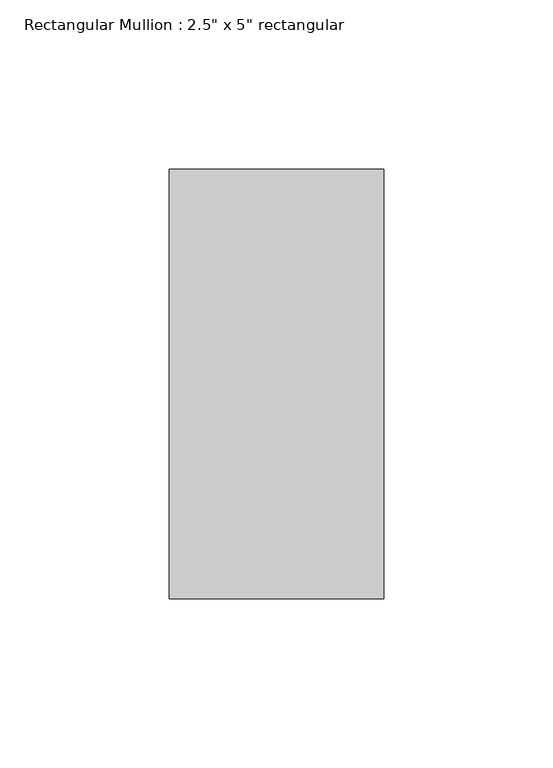
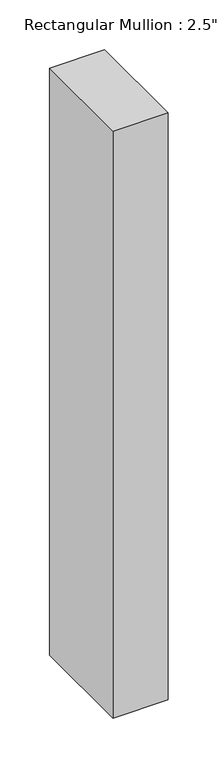
"""IFC4 building model written with IfcOpenShell, lengths in millimetres: member geometry."""

from ifc_helpers import new_model, si_unit, frame, origin, place, context, project, spatial, polyline, outline, extrude, source, transform, mapped, element, save


def member_abeaf8ac(model_context):
    return source(origin(), model_context, "Body", "SweptSolid", [
        extrude(outline(polyline([(31.75, 63.5), (31.75, -63.5), (-31.75, -63.5), (-31.75, 63.5), (31.75, 63.5)])), frame((0.0, 0.0, -717.55), z_axis=(0.0, 0.0, 1.0), x_axis=(1.0, 0.0, 0.0)), (0.0, 0.0, 1.0), 717.55),
    ])


if __name__ == "__main__":
    model = new_model("IFC4")
    model_context = context("Model", 3, world=origin())
    ifc_project = project(units=[si_unit("LENGTHUNIT", "METRE", prefix="MILLI")], contexts=[model_context])
    site = spatial("IfcSite", under=ifc_project)
    building = spatial("IfcBuilding", under=site)
    placement = place(None, origin())
    member_shape = member_abeaf8ac(model_context)
    element("IfcMember", 1, ObjectType="Rectangular Mullion : 2.5\" x 5\" rectangular", at=placement, inside=building, context=model_context, shape_type="MappedRepresentation", body=[
        mapped(member_shape, transform((0.0, 0.0, 0.0), x_axis=(1.0, 0.0, 0.0), y_axis=(0.0, 1.0, 0.0), z_axis=(0.0, 0.0, 1.0))),
    ])
    save(model, "model.ifc")

# Revit data of these elements
# Type "Rectangular Mullion : 2.5\" x 5\" rectangular"
#   built-in parameter 1007304 = 0.416667 (stored number, unit not read)
#   built-in parameter 1007301 = 0.104167 (stored number, unit not read)
#   built-in parameter 1007300 = 0.104167 (stored number, unit not read)
# Element 1 (IfcMember, "Rectangular Mullion : 2.5\" x 5\" rectangular")
#   Materials on its faces: "Aluminum"
# Materials
#   "Aluminum": class "Metal", colour RGB 247 247 247, transparency 0, Description = "Aluminum 6061", Cost = 0
